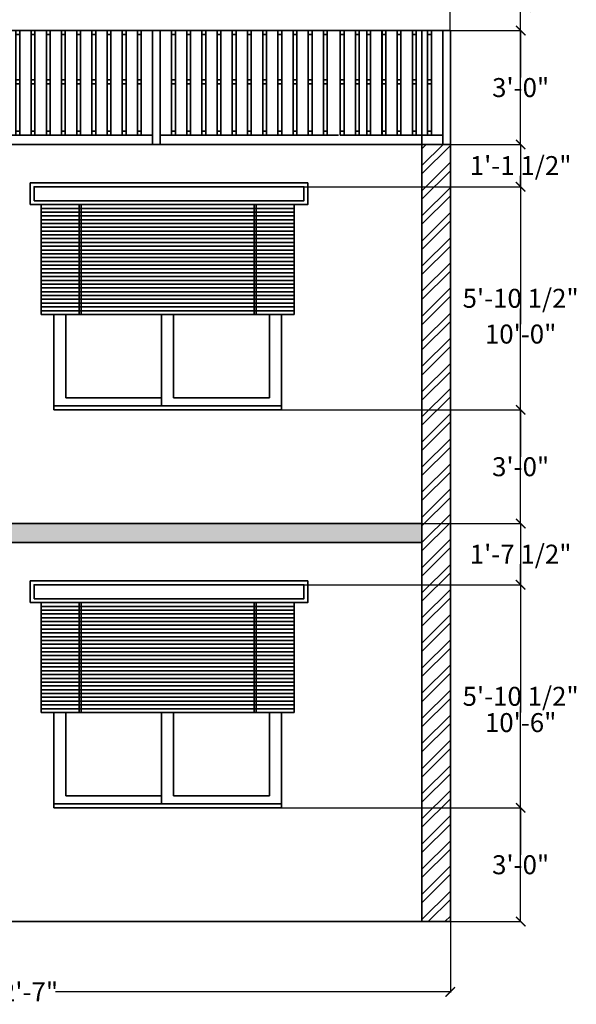
# Model space of a CAD drawing. Units: inches. Extents: x 2278 to 7495, y -71 to 1198.
# Tile 40 of 44: x 7254 to 7430, y 128 to 439. Entities that reach past the tile are written whole.
import ezdxf

# ---------------------------------------------------------------- set-up
doc = ezdxf.new("R2010")
doc.units = ezdxf.units.IN
doc.header["$MEASUREMENT"] = 0
for name, color, linetype, lineweight in [('A-ANNO-DIMS', 2, 'Continuous', 18), ('A-ANNO-TEXT', 7, 'Continuous', 25), ('A-SECT', 7, 'Continuous', 35), ('A-SECT-PATT', 8, 'Continuous', 13)]:
    doc.layers.add(name, color=color, linetype=linetype, lineweight=lineweight)
doc.styles.add('ATTR', font='romans.shx', dxfattribs={"width": 0.8, "height": 0.7})
doc.styles.get("Standard").update_dxf_attribs({"font": 'arial.ttf'})
doc.dimstyles.get("Standard").update_dxf_attribs({"dimtxt": 6, "dimasz": 3, "dimexe": 0.18, "dimexo": 0.0625, "dimgap": 0.09, "dimtad": 0, "dimtih": 1, "dimtoh": 1, "dimdec": 0, "dimzin": 0, "dimdsep": 46, "dimlunit": 3, "dimtxsty": 'Standard', "dimblk": 'ARCHTICK', "dimcen": 0.09, "dimadec": 0, "dimazin": 0, "dimtfac": 1, "dimtdec": 0, "dimtofl": 0, "dimtmove": 0, "dimatfit": 3, "dimfxl": 1, "dimtolj": 1, "dimtzin": 0, "dimarcsym": 0})

# ---------------------------------------------------------------- blocks, each defined once
blk = doc.blocks.new('Fence 2 EV')
for p, q in [((0, 60), (0, 0)), ((0.001, 60.008), (98.001, 60.008)), ((4, 0.002), (4, 60)), ((10, 60), (10, 5.002)), ((10, 58), (12, 58)), ((12, 60), (12, 5.002)), ((18, 5.002), (18, 60)), ((18, 58), (20, 58)), ((20, 60), (20, 5.002)), ((25.999, 5.002), (25.999, 60)), ((25.999, 58), (27.999, 58)), ((27.999, 60), (27.999, 5.002)), ((33.999, 5.002), (33.999, 60)), ((33.999, 58), (35.999, 58)), ((35.999, 60), (35.999, 5.002)), ((41.999, 5.002), (41.999, 60)), ((41.999, 58), (43.999, 58)), ((43.999, 60), (43.999, 5.002)), ((49.999, 5.002), (49.999, 60)), ((49.999, 58), (51.998, 58)), ((51.998, 60), (51.998, 5.002)), ((57.998, 5.002), (57.998, 60)), ((57.998, 58), (59.998, 58)), ((59.998, 60), (59.998, 5.002)), ((65.998, 5.002), (65.998, 60)), ((65.998, 58), (67.998, 58)), ((67.998, 60), (67.998, 5.002)), ((73.998, 5.002), (73.998, 60)), ((73.998, 58), (75.997, 58)), ((75.997, 60), (75.997, 5.002)), ((81.997, 5.002), (81.997, 60)), ((81.997, 58), (83.997, 58)), ((83.997, 60), (83.997, 5.002)), ((89.997, 5.002), (89.997, 60)), ((89.997, 58), (91.997, 58)), ((91.997, 60), (91.997, 5.002)), ((10, 34.001), (12, 34.001)), ((10, 32.001), (12, 32.001)), ((18, 34.001), (20, 34.001)), ((18, 32.001), (20, 32.001)), ((25.999, 34.001), (27.999, 34.001)), ((25.999, 32.001), (27.999, 32.001)), ((33.999, 34.001), (35.999, 34.001)), ((33.999, 32.001), (35.999, 32.001)), ((41.999, 34.001), (43.999, 34.001)), ((41.999, 32.001), (43.999, 32.001)), ((49.999, 34.001), (51.998, 34.001)), ((49.999, 32.001), (51.998, 32.001)), ((57.998, 34.001), (59.998, 34.001)), ((57.998, 32.001), (59.998, 32.001)), ((65.998, 34.001), (67.998, 34.001)), ((65.998, 32.001), (67.998, 32.001)), ((73.998, 34.001), (75.997, 34.001)), ((73.998, 32.001), (75.997, 32.001)), ((81.997, 34.001), (83.997, 34.001)), ((81.997, 32.001), (83.997, 32.001)), ((89.997, 34.001), (91.997, 34.001)), ((89.997, 32.001), (91.997, 32.001)), ((10, 7.002), (12, 7.002)), ((18, 7.002), (20, 7.002)), ((25.999, 7.002), (27.999, 7.002)), ((33.999, 7.002), (35.999, 7.002)), ((41.999, 7.002), (43.999, 7.002)), ((49.999, 7.002), (51.998, 7.002)), ((57.998, 7.002), (59.998, 7.002)), ((65.998, 7.002), (67.998, 7.002)), ((73.998, 7.002), (75.997, 7.002)), ((81.997, 7.002), (83.997, 7.002)), ((89.997, 7.002), (91.997, 7.002)), ((0, 0.002), (4, 0.002)), ((97.997, 5.002), (4, 5.002))]:
    blk.add_line(p, q)
at = {"style": 'ATTR', "width": 0.8, "flags": 9}
blk.add_attdef('ESTCODE', (0, 0), '', height=0.0196, dxfattribs=at)
blk = doc.blocks.new('_ArchTick')
at = {"color": 0, "linetype": 'ByBlock', "const_width": 0.15}
blk.add_lwpolyline([(-0.5, -0.5), (0.5, 0.5)], dxfattribs=at)
blk = doc.blocks.new('*D104')
at = {"layer": 'A-ANNO-DIMS', "color": 0, "lineweight": -2, "transparency": 16777216}
for p, q in [((7336.68, 189.83), (7412.55, 189.83)), ((7412.37, 189.83), (7412.37, 174.99)), ((7412.37, 153.83), (7412.37, 168.68)), ((7390.18, 153.83), (7412.55, 153.83))]:
    blk.add_line(p, q, dxfattribs=at)
at = {"layer": 'Defpoints', "color": 0, "transparency": 16777216}
for p in [(7336.62, 189.83), (7412.37, 189.83), (7390.12, 153.83)]:
    blk.add_point(p, dxfattribs=at)
at = {"layer": 'A-ANNO-DIMS', "color": 0, "lineweight": -2, "transparency": 16777216, "xscale": 3, "yscale": 3, "zscale": 3}
for p, rotation in [((7412.37, 189.83), 90), ((7412.37, 153.83), 270)]:
    blk.add_blockref('_ArchTick', p, dxfattribs=dict(at, rotation=rotation))
at = {"layer": 'A-ANNO-DIMS', "color": 0, "transparency": 16777216, "insert": (7412.37, 171.83), "char_height": 6, "attachment_point": 5}
blk.add_mtext('\\A1;3\'-0"', dxfattribs=at)
blk = doc.blocks.new('*D105')
at = {"layer": 'A-ANNO-DIMS', "color": 0, "lineweight": -2, "transparency": 16777216}
for p, q in [((7343.83, 260.48), (7412.55, 260.48)), ((7412.37, 260.48), (7412.37, 228.35)), ((7412.37, 189.83), (7412.37, 221.96)), ((7336.68, 189.83), (7412.55, 189.83))]:
    blk.add_line(p, q, dxfattribs=at)
at = {"layer": 'Defpoints', "color": 0, "transparency": 16777216}
for p in [(7343.77, 260.48), (7412.37, 260.48), (7336.62, 189.83)]:
    blk.add_point(p, dxfattribs=at)
at = {"layer": 'A-ANNO-DIMS', "color": 0, "lineweight": -2, "transparency": 16777216, "xscale": 3, "yscale": 3, "zscale": 3}
for p, rotation in [((7412.37, 260.48), 90), ((7412.37, 189.83), 270)]:
    blk.add_blockref('_ArchTick', p, dxfattribs=dict(at, rotation=rotation))
at = {"layer": 'A-ANNO-DIMS', "color": 0, "transparency": 16777216, "insert": (7412.37, 225.15), "char_height": 6, "attachment_point": 5}
blk.add_mtext('\\A1;5\'-10 1/2"', dxfattribs=at)
blk = doc.blocks.new('*D106')
at = {"layer": 'A-ANNO-DIMS', "color": 0, "lineweight": -2, "transparency": 16777216}
for p, q in [((7381.18, 279.83), (7412.55, 279.83)), ((7412.37, 279.83), (7412.37, 273.35)), ((7412.37, 260.48), (7412.37, 266.96)), ((7343.83, 260.48), (7412.55, 260.48))]:
    blk.add_line(p, q, dxfattribs=at)
at = {"layer": 'Defpoints', "color": 0, "transparency": 16777216}
for p in [(7381.12, 279.83), (7412.37, 279.83), (7343.77, 260.48)]:
    blk.add_point(p, dxfattribs=at)
at = {"layer": 'A-ANNO-DIMS', "color": 0, "lineweight": -2, "transparency": 16777216, "xscale": 3, "yscale": 3, "zscale": 3}
for p, rotation in [((7412.37, 279.83), 90), ((7412.37, 260.48), 270)]:
    blk.add_blockref('_ArchTick', p, dxfattribs=dict(at, rotation=rotation))
at = {"layer": 'A-ANNO-DIMS', "color": 0, "transparency": 16777216, "insert": (7412.37, 270.15), "char_height": 6, "attachment_point": 5}
blk.add_mtext('\\A1;1\'-7 1/2"', dxfattribs=at)
blk = doc.blocks.new('*D107')
at = {"layer": 'A-ANNO-DIMS', "color": 0, "lineweight": -2, "transparency": 16777216}
for p, q in [((7336.68, 315.83), (7412.55, 315.83)), ((7412.37, 315.83), (7412.37, 300.99)), ((7412.37, 279.83), (7412.37, 294.68)), ((7381.18, 279.83), (7412.55, 279.83))]:
    blk.add_line(p, q, dxfattribs=at)
at = {"layer": 'Defpoints', "color": 0, "transparency": 16777216}
for p in [(7336.62, 315.83), (7412.37, 315.83), (7381.12, 279.83)]:
    blk.add_point(p, dxfattribs=at)
at = {"layer": 'A-ANNO-DIMS', "color": 0, "lineweight": -2, "transparency": 16777216, "xscale": 3, "yscale": 3, "zscale": 3}
for p, rotation in [((7412.37, 315.83), 90), ((7412.37, 279.83), 270)]:
    blk.add_blockref('_ArchTick', p, dxfattribs=dict(at, rotation=rotation))
at = {"layer": 'A-ANNO-DIMS', "color": 0, "transparency": 16777216, "insert": (7412.37, 297.83), "char_height": 6, "attachment_point": 5}
blk.add_mtext('\\A1;3\'-0"', dxfattribs=at)
blk = doc.blocks.new('*D108')
at = {"layer": 'A-ANNO-DIMS', "color": 0, "lineweight": -2, "transparency": 16777216}
for p, q in [((7343.83, 386.48), (7412.55, 386.48)), ((7412.37, 386.48), (7412.37, 354.35)), ((7412.37, 315.83), (7412.37, 347.96)), ((7336.68, 315.83), (7412.55, 315.83))]:
    blk.add_line(p, q, dxfattribs=at)
at = {"layer": 'Defpoints', "color": 0, "transparency": 16777216}
for p in [(7343.77, 386.48), (7412.37, 386.48), (7336.62, 315.83)]:
    blk.add_point(p, dxfattribs=at)
at = {"layer": 'A-ANNO-DIMS', "color": 0, "lineweight": -2, "transparency": 16777216, "xscale": 3, "yscale": 3, "zscale": 3}
for p, rotation in [((7412.37, 386.48), 90), ((7412.37, 315.83), 270)]:
    blk.add_blockref('_ArchTick', p, dxfattribs=dict(at, rotation=rotation))
at = {"layer": 'A-ANNO-DIMS', "color": 0, "transparency": 16777216, "insert": (7412.37, 351.15), "char_height": 6, "attachment_point": 5}
blk.add_mtext('\\A1;5\'-10 1/2"', dxfattribs=at)
blk = doc.blocks.new('*D109')
at = {"layer": 'A-ANNO-DIMS', "color": 0, "lineweight": -2, "transparency": 16777216}
for p, q in [((7390.18, 399.83), (7412.55, 399.83)), ((7412.37, 399.83), (7412.37, 396.35)), ((7412.37, 386.48), (7412.37, 389.96)), ((7343.83, 386.48), (7412.55, 386.48))]:
    blk.add_line(p, q, dxfattribs=at)
at = {"layer": 'Defpoints', "color": 0, "transparency": 16777216}
for p in [(7390.12, 399.83), (7412.37, 399.83), (7343.77, 386.48)]:
    blk.add_point(p, dxfattribs=at)
at = {"layer": 'A-ANNO-DIMS', "color": 0, "lineweight": -2, "transparency": 16777216, "xscale": 3, "yscale": 3, "zscale": 3}
for p, rotation in [((7412.37, 399.83), 90), ((7412.37, 386.48), 270)]:
    blk.add_blockref('_ArchTick', p, dxfattribs=dict(at, rotation=rotation))
at = {"layer": 'A-ANNO-DIMS', "color": 0, "transparency": 16777216, "insert": (7412.37, 393.16), "char_height": 6, "attachment_point": 5}
blk.add_mtext('\\A1;1\'-1 1/2"', dxfattribs=at)
blk = doc.blocks.new('*D110')
at = {"layer": 'A-ANNO-DIMS', "color": 0, "lineweight": -2, "transparency": 16777216}
for p, q in [((7390.18, 435.89), (7412.55, 435.89)), ((7412.37, 435.89), (7412.37, 421.02)), ((7412.37, 399.83), (7412.37, 414.71)), ((7390.18, 399.83), (7412.55, 399.83))]:
    blk.add_line(p, q, dxfattribs=at)
at = {"layer": 'Defpoints', "color": 0, "transparency": 16777216}
for p in [(7390.11, 435.89), (7412.37, 435.89), (7390.12, 399.83)]:
    blk.add_point(p, dxfattribs=at)
at = {"layer": 'A-ANNO-DIMS', "color": 0, "lineweight": -2, "transparency": 16777216, "xscale": 3, "yscale": 3, "zscale": 3}
for p, rotation in [((7412.37, 435.89), 90), ((7412.37, 399.83), 270)]:
    blk.add_blockref('_ArchTick', p, dxfattribs=dict(at, rotation=rotation))
at = {"layer": 'A-ANNO-DIMS', "color": 0, "transparency": 16777216, "insert": (7412.37, 417.86), "char_height": 6, "attachment_point": 5}
blk.add_mtext('\\A1;3\'-0"', dxfattribs=at)
blk = doc.blocks.new('*D111')
at = {"layer": 'A-ANNO-DIMS', "color": 0, "lineweight": -2, "transparency": 16777216}
for p, q in [((7381.18, 279.83), (7412.55, 279.83)), ((7412.37, 279.83), (7412.37, 219.99)), ((7412.37, 153.83), (7412.37, 213.68)), ((7390.18, 153.83), (7412.55, 153.83))]:
    blk.add_line(p, q, dxfattribs=at)
at = {"layer": 'Defpoints', "color": 0, "transparency": 16777216}
for p in [(7381.12, 279.83), (7412.37, 279.83), (7390.12, 153.83)]:
    blk.add_point(p, dxfattribs=at)
at = {"layer": 'A-ANNO-DIMS', "color": 0, "lineweight": -2, "transparency": 16777216, "xscale": 3, "yscale": 3, "zscale": 3}
for p, rotation in [((7412.37, 279.83), 90), ((7412.37, 153.83), 270)]:
    blk.add_blockref('_ArchTick', p, dxfattribs=dict(at, rotation=rotation))
at = {"layer": 'A-ANNO-DIMS', "color": 0, "transparency": 16777216, "insert": (7412.37, 216.83), "char_height": 6, "attachment_point": 5}
blk.add_mtext('\\A1;10\'-6"', dxfattribs=at)
blk = doc.blocks.new('*D112')
at = {"layer": 'A-ANNO-DIMS', "color": 0, "lineweight": -2, "transparency": 16777216}
for p, q in [((7390.18, 399.83), (7412.55, 399.83)), ((7412.37, 399.83), (7412.37, 342.99)), ((7412.37, 279.83), (7412.37, 336.68)), ((7381.18, 279.83), (7412.55, 279.83))]:
    blk.add_line(p, q, dxfattribs=at)
at = {"layer": 'Defpoints', "color": 0, "transparency": 16777216}
for p in [(7390.12, 399.83), (7412.37, 399.83), (7381.12, 279.83)]:
    blk.add_point(p, dxfattribs=at)
at = {"layer": 'A-ANNO-DIMS', "color": 0, "lineweight": -2, "transparency": 16777216, "xscale": 3, "yscale": 3, "zscale": 3}
for p, rotation in [((7412.37, 399.83), 90), ((7412.37, 279.83), 270)]:
    blk.add_blockref('_ArchTick', p, dxfattribs=dict(at, rotation=rotation))
at = {"layer": 'A-ANNO-DIMS', "color": 0, "transparency": 16777216, "insert": (7412.37, 339.83), "char_height": 6, "attachment_point": 5}
blk.add_mtext('\\A1;10\'-0"', dxfattribs=at)
blk = doc.blocks.new('*D113')
at = {"layer": 'A-ANNO-DIMS', "color": 0, "lineweight": -2, "transparency": 16777216}
for p, q in [((7119.18, 489.83), (7412.55, 489.83)), ((7412.37, 489.83), (7412.37, 447.99)), ((7412.37, 399.83), (7412.37, 441.68)), ((7119.18, 399.83), (7412.55, 399.83))]:
    blk.add_line(p, q, dxfattribs=at)
at = {"layer": 'Defpoints', "color": 0, "transparency": 16777216}
for p in [(7119.12, 489.83), (7412.37, 489.83), (7119.12, 399.83)]:
    blk.add_point(p, dxfattribs=at)
at = {"layer": 'A-ANNO-DIMS', "color": 0, "lineweight": -2, "transparency": 16777216, "xscale": 3, "yscale": 3, "zscale": 3}
for p, rotation in [((7412.37, 489.83), 90), ((7412.37, 399.83), 270)]:
    blk.add_blockref('_ArchTick', p, dxfattribs=dict(at, rotation=rotation))
at = {"layer": 'A-ANNO-DIMS', "color": 0, "transparency": 16777216, "insert": (7412.37, 444.83), "char_height": 6, "attachment_point": 5}
blk.add_mtext('\\A1;7\'-6"', dxfattribs=at)
blk = doc.blocks.new('*D120')
at = {"layer": 'A-ANNO-DIMS', "color": 0, "lineweight": -2, "transparency": 16777216}
for p, q in [((7119.12, 161.77), (7119.12, 131.4)), ((7390.12, 153.77), (7390.12, 131.4)), ((7119.12, 131.58), (7244.17, 131.58)), ((7390.12, 131.58), (7265.06, 131.58))]:
    blk.add_line(p, q, dxfattribs=at)
at = {"layer": 'Defpoints', "color": 0, "transparency": 16777216}
for p in [(7119.12, 161.83), (7390.12, 153.83), (7390.12, 131.58)]:
    blk.add_point(p, dxfattribs=at)
at = {"layer": 'A-ANNO-DIMS', "color": 0, "lineweight": -2, "transparency": 16777216, "xscale": 3, "yscale": 3, "zscale": 3, "rotation": 180}
blk.add_blockref('_ArchTick', (7119.12, 131.58), dxfattribs=at)
at = {"layer": 'A-ANNO-DIMS', "color": 0, "lineweight": -2, "transparency": 16777216, "xscale": 3, "yscale": 3, "zscale": 3}
blk.add_blockref('_ArchTick', (7390.12, 131.58), dxfattribs=at)
at = {"layer": 'A-ANNO-DIMS', "color": 0, "transparency": 16777216, "insert": (7254.62, 131.58), "char_height": 6, "attachment_point": 5}
blk.add_mtext('\\A1;22\'-7"', dxfattribs=at)
blk = doc.blocks.new('*D122')
at = {"layer": 'A-ANNO-DIMS', "color": 0, "lineweight": -2, "transparency": 16777216}
for p, q in [((7119.12, 489.9), (7119.12, 512.26)), ((7119.12, 512.08), (7244.17, 512.08)), ((7390.11, 512.08), (7265.06, 512.08)), ((7390.11, 435.95), (7390.11, 512.26))]:
    blk.add_line(p, q, dxfattribs=at)
at = {"layer": 'Defpoints', "color": 0, "transparency": 16777216}
for p in [(7390.11, 512.08), (7119.12, 489.83), (7390.11, 435.89)]:
    blk.add_point(p, dxfattribs=at)
at = {"layer": 'A-ANNO-DIMS', "color": 0, "lineweight": -2, "transparency": 16777216, "xscale": 3, "yscale": 3, "zscale": 3, "rotation": 180}
blk.add_blockref('_ArchTick', (7119.12, 512.08), dxfattribs=at)
at = {"layer": 'A-ANNO-DIMS', "color": 0, "lineweight": -2, "transparency": 16777216, "xscale": 3, "yscale": 3, "zscale": 3}
blk.add_blockref('_ArchTick', (7390.11, 512.08), dxfattribs=at)
at = {"layer": 'A-ANNO-DIMS', "color": 0, "transparency": 16777216, "insert": (7254.61, 512.08), "char_height": 6, "attachment_point": 5}
blk.add_mtext('\\A1;22\'-7"', dxfattribs=at)

msp = doc.modelspace()

# ---------------------------------------------------------------- hatches: boundary and pattern name
at = {"layer": 'A-SECT-PATT', "transparency": 33554687}
h = msp.add_hatch(dxfattribs=at)
h.set_pattern_fill('ANSI32', color=256, scale=15)
h.set_pattern_definition([(45, (0, 155.58), (-3.9774756, 3.9774756), []), (45, (2.6517, 155.58), (-3.9774756, 3.9774756), [])])
h.paths.add_polyline_path([(6996.12, 489.83), (6987.12, 489.83), (6987.12, 153.83), (6996.12, 153.83)])
h.paths.add_polyline_path([(7390.12, 399.83), (7381.12, 399.83), (7381.12, 153.83), (7390.12, 153.83)])
h.paths.add_polyline_path([(7119.12, 483.83), (7119.12, 489.83), (7113.12, 489.83), (7113.12, 399.83), (7119.12, 399.83)])
h = msp.add_hatch(dxfattribs=at)
h.set_pattern_fill('AR-CONC', color=256, scale=0.8)
h.set_pattern_definition([(50, (0, 0), (5.7380815, -0.502017), [0.6, -6.6]), (355, (0, 0), (-1.1100107, 6.017537), [0.48, -5.28]), (100.451444, (0.478, -0.042), (4.6280708, 5.51552), [0.5099215, -5.609137]), (46.1842, (0, 1.6), (8.5379306, -1.324154), [0.9, -9.9]), (96.63564, (0.7115, 1.49), (7.477296, 7.792949), [0.764883, -8.41371]), (351.18416, (0, 1.6), (7.477296, 7.792949), [0.72, -7.92]), (21, (0.8, 1.2), (4.7752564, -3.220951), [0.6, -6.6]), (326, (0.8, 1.2), (1.9465227, 5.8012004), [0.48, -5.28]), (71.451445, (1.198, 0.9316), (6.721779, 2.5802492), [0.5099215, -5.609137]), (37.5, (0, 0), (0.09727884, 2.66315083), [0, -5.216, 0, -5.36, 0, -5.3]), (7.5, (0, 0), (2.1045563, 3.1552937), [0, -3.056, 0, -5.096, 0, -2.02]), (327.5, (-1.784, 0), (4.2705795, -0.180439), [0, -2, 0, -6.24, 0, -8.28]), (317.5, (-2.584, 0), (4.6654894, 0.8008399), [0, -2.6, 0, -4.144, 0, -5.88])])
h.paths.add_polyline_path([(7381.12, 279.83), (6996.12, 279.83), (6996.12, 273.83), (7131.12, 273.83), (7143.12, 273.83), (7167.12, 273.83), (7381.12, 273.83)])

# ---------------------------------------------------------------- linework, layer by layer
at = {"layer": 'A-SECT'}
for p, q in [((7355.26, 435.88), (7354.74, 435.89)), ((7390.11, 435.89), (7355.26, 435.89)), ((7355.26, 435.88), (7355.26, 402.84)), ((7356.46, 434.68), (7355.26, 434.68)), ((7356.46, 402.84), (7356.46, 435.88)), ((7360.04, 402.84), (7360.04, 435.88)), ((7360.07, 434.68), (7360.04, 434.68)), ((7360.07, 402.84), (7360.07, 435.88)), ((7360.07, 435.88), (7360.07, 402.84)), ((7361.27, 434.68), (7360.07, 434.68)), ((7361.27, 402.84), (7361.27, 435.88)), ((7363.65, 435.88), (7363.65, 402.84)), ((7364.85, 434.68), (7363.65, 434.68)), ((7363.68, 435.88), (7363.68, 402.84)), ((7364.88, 434.68), (7363.68, 434.68)), ((7364.85, 402.84), (7364.85, 435.88)), ((7364.88, 402.84), (7364.88, 435.88)), ((7368.45, 435.88), (7368.45, 402.84)), ((7369.66, 434.68), (7368.45, 434.68)), ((7368.49, 435.88), (7368.49, 402.84)), ((7369.69, 434.68), (7368.49, 434.68)), ((7369.66, 402.84), (7369.66, 435.88)), ((7369.69, 402.84), (7369.69, 435.88)), ((7373.29, 435.88), (7373.29, 402.84)), ((7374.49, 434.68), (7373.29, 434.68)), ((7374.49, 402.84), (7374.49, 435.88)), ((7378.1, 435.88), (7378.1, 402.84)), ((7379.3, 434.68), (7378.1, 434.68)), ((7379.3, 402.84), (7379.3, 435.88)), ((7381.12, 153.83), (7381.12, 435.89)), ((7382.91, 435.88), (7382.91, 402.84)), ((7384.11, 434.68), (7382.91, 434.68)), ((7384.11, 435.88), (7384.11, 402.84)), ((7387.71, 399.83), (7387.71, 435.88)), ((7390.12, 435.88), (7390.12, 399.83)), ((7356.46, 420.26), (7355.26, 420.26)), ((7356.46, 419.06), (7355.26, 419.06)), ((7361.27, 420.26), (7360.07, 420.26)), ((7361.27, 419.06), (7360.07, 419.06)), ((7364.85, 420.26), (7363.65, 420.26)), ((7364.85, 419.06), (7363.65, 419.06)), ((7364.88, 420.26), (7363.68, 420.26)), ((7364.88, 419.06), (7363.68, 419.06)), ((7369.66, 420.26), (7368.45, 420.26)), ((7369.66, 419.06), (7368.45, 419.06)), ((7369.69, 420.26), (7368.49, 420.26)), ((7369.69, 419.06), (7368.49, 419.06)), ((7374.49, 420.26), (7373.29, 420.26)), ((7374.49, 419.06), (7373.29, 419.06)), ((7379.3, 420.26), (7378.1, 420.26)), ((7379.3, 419.06), (7378.1, 419.06)), ((7384.11, 420.26), (7382.91, 420.26)), ((7384.11, 419.06), (7382.91, 419.06)), ((7356.46, 404.04), (7355.26, 404.04)), ((7355.26, 402.84), (7387.71, 402.84)), ((7361.27, 404.04), (7360.07, 404.04)), ((7364.85, 404.04), (7363.65, 404.04)), ((7364.88, 404.04), (7363.68, 404.04)), ((7369.66, 404.04), (7368.45, 404.04)), ((7369.69, 404.04), (7368.49, 404.04)), ((7374.49, 404.04), (7373.29, 404.04)), ((7379.3, 404.04), (7378.1, 404.04)), ((7384.11, 404.04), (7382.91, 404.04)), ((6996.12, 399.83), (7390.12, 399.83)), ((7390.12, 399.83), (7387.71, 399.83)), ((7390.12, 153.83), (7390.12, 399.83)), ((7260.62, 380.83), (7340.62, 380.83)), ((7260.62, 380.83), (7260.62, 346.03)), ((7272.62, 380.83), (7272.62, 346.03)), ((7272.62, 380.83), (7272.62, 347.23)), ((7272.62, 380.83), (7272.62, 347.23)), ((7272.62, 380.83), (7272.62, 347.23)), ((7273.22, 380.83), (7273.22, 346.03)), ((7273.22, 380.83), (7273.22, 347.23)), ((7273.22, 380.83), (7273.22, 347.23)), ((7273.22, 380.83), (7273.22, 347.23)), ((7328.02, 380.83), (7328.02, 346.03)), ((7328.02, 380.83), (7328.02, 347.23)), ((7328.02, 380.83), (7328.02, 347.23)), ((7328.02, 380.83), (7328.02, 347.23)), ((7328.62, 380.83), (7328.62, 346.03)), ((7328.62, 380.83), (7328.62, 347.23)), ((7328.62, 380.83), (7328.62, 347.23)), ((7328.62, 380.83), (7328.62, 347.23)), ((7340.62, 346.03), (7340.62, 380.83)), ((7260.62, 379.63), (7340.62, 379.63)), ((7260.62, 378.43), (7340.62, 378.43)), ((7260.62, 377.23), (7340.62, 377.23)), ((7260.62, 376.03), (7340.62, 376.03)), ((7260.62, 374.83), (7340.62, 374.83)), ((7260.62, 373.63), (7340.62, 373.63)), ((7260.62, 372.43), (7340.62, 372.43)), ((7260.62, 371.23), (7340.62, 371.23)), ((7260.62, 370.03), (7340.62, 370.03)), ((7260.62, 368.83), (7340.62, 368.83)), ((7260.62, 367.63), (7340.62, 367.63)), ((7260.62, 366.43), (7340.62, 366.43)), ((7260.62, 365.23), (7340.62, 365.23)), ((7260.62, 364.03), (7340.62, 364.03)), ((7260.62, 362.83), (7340.62, 362.83)), ((7260.62, 361.63), (7340.62, 361.63)), ((7260.62, 360.43), (7340.62, 360.43)), ((7260.62, 359.23), (7340.62, 359.23)), ((7260.62, 358.03), (7340.62, 358.03)), ((7260.62, 356.83), (7340.62, 356.83)), ((7260.62, 355.63), (7340.62, 355.63)), ((7260.62, 354.43), (7340.62, 354.43)), ((7260.62, 353.23), (7340.62, 353.23)), ((7260.62, 352.03), (7340.62, 352.03)), ((7260.62, 350.83), (7340.62, 350.83)), ((7260.62, 349.63), (7340.62, 349.63)), ((7260.62, 348.43), (7340.62, 348.43)), ((7260.62, 347.23), (7340.62, 347.23)), ((7260.62, 346.03), (7340.62, 346.03)), ((7264.62, 315.83), (7264.62, 346.03)), ((7264.62, 315.83), (7264.62, 346.03)), ((7264.62, 346.03), (7264.62, 315.83)), ((7264.62, 346.03), (7264.62, 317.12)), ((7264.62, 346.03), (7264.62, 317.12)), ((7268.4, 346.03), (7268.4, 319.69)), ((7268.4, 346.03), (7268.4, 319.69)), ((7298.72, 317.12), (7298.72, 346.03)), ((7298.72, 317.12), (7298.72, 346.03)), ((7302.51, 346.03), (7302.51, 319.69)), ((7302.51, 346.03), (7302.51, 319.69)), ((7332.83, 319.69), (7332.83, 346.03)), ((7332.83, 319.69), (7332.83, 346.03)), ((7336.62, 346.03), (7336.62, 317.12)), ((7336.62, 346.03), (7336.62, 317.12)), ((7336.62, 346.03), (7336.62, 315.83)), ((7336.62, 346.03), (7336.62, 315.83)), ((7336.62, 346.03), (7336.62, 315.83)), ((7336.62, 317.12), (7336.62, 346.03)), ((7268.4, 319.69), (7298.72, 319.69)), ((7268.4, 319.69), (7298.72, 319.69)), ((7302.51, 319.69), (7332.83, 319.69)), ((7302.51, 319.69), (7332.83, 319.69)), ((7264.62, 317.12), (7336.62, 317.12)), ((7264.62, 317.12), (7336.62, 317.12)), ((7336.62, 315.83), (7264.62, 315.83)), ((7336.62, 315.83), (7264.62, 315.83)), ((7336.62, 315.83), (7264.62, 315.83)), ((7264.62, 315.83), (7264.62, 315.83)), ((7336.62, 315.83), (7264.62, 315.83)), ((7336.62, 317.12), (7298.72, 317.12)), ((6996.12, 279.83), (7381.12, 279.83)), ((7167.12, 273.83), (7381.12, 273.83)), ((7260.62, 254.83), (7340.62, 254.83)), ((7260.62, 254.83), (7260.62, 220.03)), ((7260.62, 253.63), (7340.62, 253.63)), ((7272.62, 254.83), (7272.62, 220.03)), ((7272.62, 254.83), (7272.62, 221.23)), ((7272.62, 254.83), (7272.62, 221.23)), ((7272.62, 254.83), (7272.62, 221.23)), ((7273.22, 254.83), (7273.22, 220.03)), ((7273.22, 254.83), (7273.22, 221.23)), ((7273.22, 254.83), (7273.22, 221.23)), ((7273.22, 254.83), (7273.22, 221.23)), ((7328.02, 254.83), (7328.02, 220.03)), ((7328.02, 254.83), (7328.02, 221.23)), ((7328.02, 254.83), (7328.02, 221.23)), ((7328.02, 254.83), (7328.02, 221.23)), ((7328.62, 254.83), (7328.62, 220.03)), ((7328.62, 254.83), (7328.62, 221.23)), ((7328.62, 254.83), (7328.62, 221.23)), ((7328.62, 254.83), (7328.62, 221.23)), ((7340.62, 220.03), (7340.62, 254.83)), ((7260.62, 252.43), (7340.62, 252.43)), ((7260.62, 251.23), (7340.62, 251.23)), ((7260.62, 250.03), (7340.62, 250.03)), ((7260.62, 248.83), (7340.62, 248.83)), ((7260.62, 247.63), (7340.62, 247.63)), ((7260.62, 246.43), (7340.62, 246.43)), ((7260.62, 245.23), (7340.62, 245.23)), ((7260.62, 244.03), (7340.62, 244.03)), ((7260.62, 242.83), (7340.62, 242.83)), ((7260.62, 241.63), (7340.62, 241.63)), ((7260.62, 240.43), (7340.62, 240.43)), ((7260.62, 239.23), (7340.62, 239.23)), ((7260.62, 238.03), (7340.62, 238.03)), ((7260.62, 236.83), (7340.62, 236.83)), ((7260.62, 235.63), (7340.62, 235.63)), ((7260.62, 234.43), (7340.62, 234.43)), ((7260.62, 233.23), (7340.62, 233.23)), ((7260.62, 232.03), (7340.62, 232.03)), ((7260.62, 230.83), (7340.62, 230.83)), ((7260.62, 229.63), (7340.62, 229.63)), ((7260.62, 228.43), (7340.62, 228.43)), ((7260.62, 227.23), (7340.62, 227.23)), ((7260.62, 226.03), (7340.62, 226.03)), ((7260.62, 224.83), (7340.62, 224.83)), ((7260.62, 223.63), (7340.62, 223.63)), ((7260.62, 222.43), (7340.62, 222.43)), ((7260.62, 221.23), (7340.62, 221.23)), ((7260.62, 220.03), (7340.62, 220.03)), ((7264.62, 189.83), (7264.62, 220.03)), ((7264.62, 189.83), (7264.62, 220.03)), ((7264.62, 220.03), (7264.62, 189.83)), ((7264.62, 220.03), (7264.62, 191.12)), ((7264.62, 220.03), (7264.62, 191.12)), ((7268.4, 220.03), (7268.4, 193.69)), ((7268.4, 220.03), (7268.4, 193.69)), ((7298.72, 191.12), (7298.72, 220.03)), ((7298.72, 191.12), (7298.72, 220.03)), ((7302.51, 220.03), (7302.51, 193.69)), ((7302.51, 220.03), (7302.51, 193.69)), ((7332.83, 193.69), (7332.83, 220.03)), ((7332.83, 193.69), (7332.83, 220.03)), ((7336.62, 220.03), (7336.62, 191.12)), ((7336.62, 220.03), (7336.62, 191.12)), ((7336.62, 220.03), (7336.62, 189.83)), ((7336.62, 220.03), (7336.62, 189.83)), ((7336.62, 220.03), (7336.62, 189.83)), ((7336.62, 191.12), (7336.62, 220.03)), ((7268.4, 193.69), (7298.72, 193.69)), ((7268.4, 193.69), (7298.72, 193.69)), ((7302.51, 193.69), (7332.83, 193.69)), ((7302.51, 193.69), (7332.83, 193.69)), ((7264.62, 191.12), (7336.62, 191.12)), ((7264.62, 191.12), (7336.62, 191.12)), ((7336.62, 191.12), (7298.72, 191.12)), ((7336.62, 189.83), (7264.62, 189.83)), ((7336.62, 189.83), (7264.62, 189.83)), ((7336.62, 189.83), (7264.62, 189.83)), ((7264.62, 189.83), (7264.62, 189.83)), ((7336.62, 189.83), (7264.62, 189.83)), ((6987.12, 153.83), (7390.12, 153.83))]:
    msp.add_line(p, q, dxfattribs=at)
for points in [[(7257.13, 380.83), (7344.97, 380.83), (7344.97, 387.68), (7257.13, 387.68)], [(7258.33, 382.03), (7343.77, 382.03), (7343.77, 386.48), (7258.33, 386.48)], [(7257.13, 254.83), (7344.97, 254.83), (7344.97, 261.68), (7257.13, 261.68)], [(7258.33, 256.03), (7343.77, 256.03), (7343.77, 260.48), (7258.33, 260.48)]]:
    msp.add_lwpolyline(points, close=True, dxfattribs=at)

# ---------------------------------------------------------------- block references
at = {"layer": 'A-SECT', "xscale": 0.600830084310023, "yscale": 0.600830084310023, "zscale": 0.600830084310023}
for p in [(7236.98, 399.83), (7295.86, 399.83)]:
    msp.add_blockref('Fence 2 EV', p, dxfattribs=at)

# ---------------------------------------------------------------- texts
at = {"layer": 'A-ANNO-TEXT', "style": 'ATTR', "width": 0.8, "flags": 9}
msp.add_attdef('ESTCODE', (7390.12, 399.83), '', height=0.0118, dxfattribs=at)

# ---------------------------------------------------------------- dimensions: what is measured, and where the dimension line sits
at = {"layer": 'A-ANNO-DIMS'}
for base, p1, p2, picture, middle in [((7390.11, 512.08), (7119.12, 489.83), (7390.11, 435.89), '*D122', (7254.61, 512.08)), ((7390.12, 131.58), (7119.12, 161.83), (7390.12, 153.83), '*D120', (7254.62, 131.58))]:
    dim = msp.add_linear_dim(base=base, p1=p1, p2=p2, dimstyle='Standard', override={"dimdec": 1, "dimlfac": 1, "dimrnd": 0, "dimzin": 1, "dimdsep": 46, "dimlunit": 4, "dimfrac": 2}, dxfattribs=at)
    dim.commit()
    dim.dimension.update_dxf_attribs({"geometry": picture, "text_midpoint": middle})
for base, p1, p2, picture, middle in [((7412.37, 489.83), (7119.12, 399.83), (7119.12, 489.83), '*D113', (7412.37, 444.83)), ((7412.37, 435.89), (7390.12, 399.83), (7390.11, 435.89), '*D110', (7412.37, 417.86)), ((7412.3653, 399.8341), (7343.768, 386.4769), (7390.1153, 399.8341), '*D109', (7412.3653, 393.1555)), ((7412.37, 399.83), (7381.12, 279.83), (7390.12, 399.83), '*D112', (7412.37, 339.83)), ((7412.3653, 386.4769), (7336.6153, 315.8329), (7343.768, 386.4769), '*D108', (7412.3653, 351.1549)), ((7412.37, 315.83), (7381.12, 279.83), (7336.62, 315.83), '*D107', (7412.37, 297.83)), ((7412.3653, 279.8329), (7343.768, 260.4769), (7381.1153, 279.8329), '*D106', (7412.3653, 270.1549)), ((7412.37, 279.83), (7390.12, 153.83), (7381.12, 279.83), '*D111', (7412.37, 216.83)), ((7412.3653, 260.4769), (7336.6153, 189.8329), (7343.768, 260.4769), '*D105', (7412.3653, 225.1549)), ((7412.37, 189.83), (7390.12, 153.83), (7336.62, 189.83), '*D104', (7412.37, 171.83))]:
    dim = msp.add_linear_dim(base=base, p1=p1, p2=p2, angle=90, dimstyle='Standard', override={"dimdec": 1, "dimlfac": 1, "dimrnd": 0, "dimzin": 1, "dimdsep": 46, "dimlunit": 4, "dimfrac": 2}, dxfattribs=at)
    dim.commit()
    dim.dimension.update_dxf_attribs({"geometry": picture, "text_midpoint": middle})

doc.saveas('drawing.dxf')
